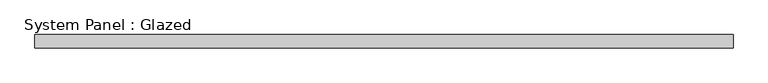
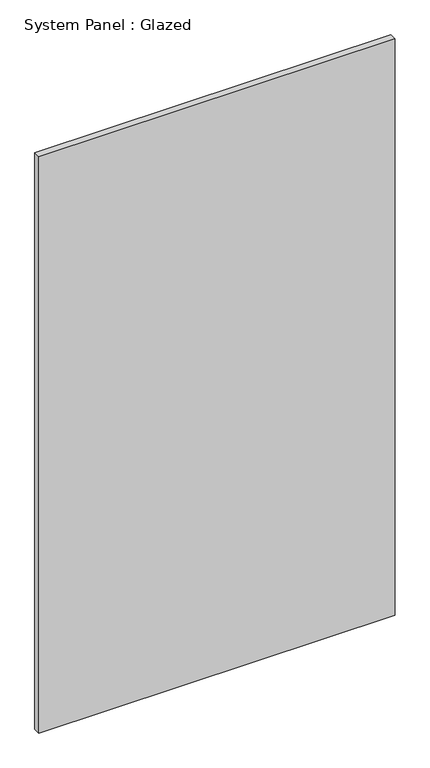
"""IFC4 building model written with IfcOpenShell, lengths in millimetres: plate geometry, System Panel : Glazed."""

from ifc_helpers import new_model, si_unit, origin, origin_with_axes, place, context, project, spatial, polyline, outline, extrude, source, transform, mapped, element, save


def system_panel_glazed_febae1d4(model_context):
    return source(origin(), model_context, "Body", "SweptSolid", [
        extrude(outline(polyline([(676.275, 19.05), (-676.275, 19.05), (-676.275, 44.45), (676.275, 44.45), (676.275, 19.05)])), origin_with_axes(), (0.0, 0.0, 1.0), 2311.4),
    ])


if __name__ == "__main__":
    model = new_model("IFC4")
    model_context = context("Model", 3, world=origin())
    ifc_project = project(units=[si_unit("LENGTHUNIT", "METRE", prefix="MILLI")], contexts=[model_context])
    site = spatial("IfcSite", under=ifc_project)
    building = spatial("IfcBuilding", under=site)
    placement = place(None, origin())
    system_panel_glazed_shape = system_panel_glazed_febae1d4(model_context)
    element("IfcPlate", 1, ObjectType="System Panel : Glazed", at=placement, inside=building, context=model_context, shape_type="MappedRepresentation", body=[
        mapped(system_panel_glazed_shape, transform((0.0, 0.0, 0.0), x_axis=(1.0, 0.0, 0.0), y_axis=(0.0, 1.0, 0.0), z_axis=(0.0, 0.0, 1.0))),
    ])
    save(model, "model.ifc")

# Revit data of these elements
# Type "System Panel : Glazed"
#   Construction Type Id = "GSP4R"
#   Analytic Construction = "1/8 in Pilkington single glazing"
#   Visual Light Transmittance = 0.9
#   Solar Heat Gain Coefficient = 0.86
#   Heat Transfer Coefficient (U) = 1.18115 BTU/(h·ft²·°F)
# Element 1 (IfcPlate, "System Panel : Glazed")
#   Materials on its faces: "Glass"
# Materials
#   "Glass": class "Glass", colour RGB 0 128 192, transparency 0.75, Description = "Soda Lime Glass", Cost = 0
